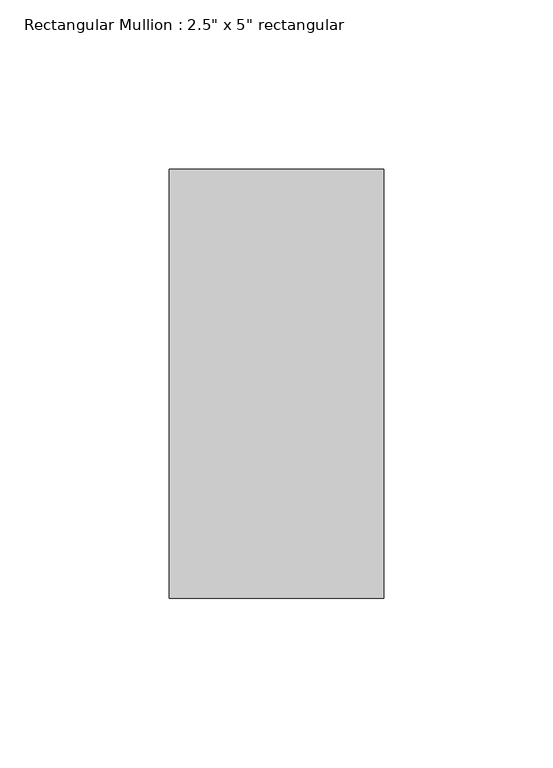
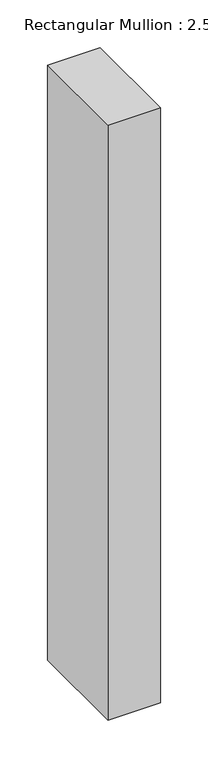
"""IFC4 building model written with IfcOpenShell, lengths in millimetres: member geometry."""

from ifc_helpers import new_model, si_unit, frame, origin, place, context, project, spatial, polyline, outline, extrude, source, transform, mapped, element, save


def member_aa870034(model_context):
    return source(origin(), model_context, "Body", "SweptSolid", [
        extrude(outline(polyline([(0.0, 63.5), (0.0, -63.5), (-63.5, -63.5), (-63.5, 63.5), (0.0, 63.5)])), frame((0.0, 0.0, -762.0), z_axis=(0.0, 0.0, 1.0), x_axis=(1.0, 0.0, 0.0)), (0.0, 0.0, 1.0), 762.0),
    ])


if __name__ == "__main__":
    model = new_model("IFC4")
    model_context = context("Model", 3, world=origin())
    ifc_project = project(units=[si_unit("LENGTHUNIT", "METRE", prefix="MILLI")], contexts=[model_context])
    site = spatial("IfcSite", under=ifc_project)
    building = spatial("IfcBuilding", under=site)
    placement = place(None, origin())
    member_shape = member_aa870034(model_context)
    element("IfcMember", 1, ObjectType="Rectangular Mullion : 2.5\" x 5\" rectangular", at=placement, inside=building, context=model_context, shape_type="MappedRepresentation", body=[
        mapped(member_shape, transform((0.0, 0.0, 0.0), x_axis=(1.0, 0.0, 0.0), y_axis=(0.0, 1.0, 0.0), z_axis=(0.0, 0.0, 1.0))),
    ])
    save(model, "model.ifc")

# Revit data of these elements
# Type "Rectangular Mullion : 2.5\" x 5\" rectangular"
#   built-in parameter 1007304 = 0.416667 (stored number, unit not read)
#   built-in parameter 1007301 = 0.104167 (stored number, unit not read)
#   built-in parameter 1007300 = 0.104167 (stored number, unit not read)
# Element 1 (IfcMember, "Rectangular Mullion : 2.5\" x 5\" rectangular")
#   Materials on its faces: "Aluminum"
# Materials
#   "Aluminum": class "Metal", colour RGB 247 247 247, transparency 0, Description = "Aluminum 6061", Cost = 0
